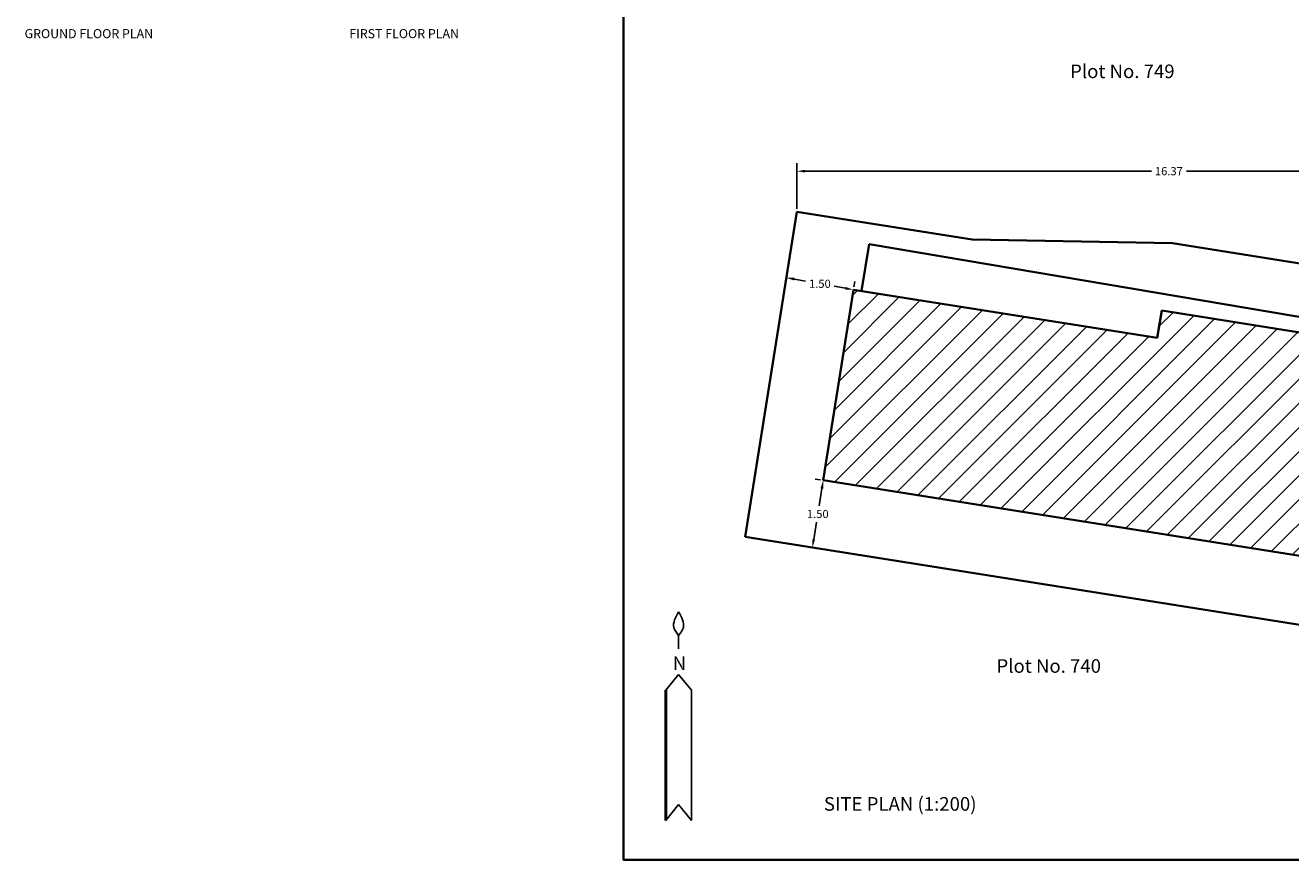
# Model space of a CAD drawing. Units: metres. Extents: x 8.1 to 56.2, y -9.3 to 36.3.
# Tile 1 of 6: x 9.4 to 37.2, y -9.3 to 9.1. Entities that reach past the tile are written whole.
import ezdxf

# ---------------------------------------------------------------- set-up
doc = ezdxf.new("R2010")
doc.units = ezdxf.units.M
doc.header["$LTSCALE"] = 0.01
doc.header["$MEASUREMENT"] = 0
for name, color, linetype, lineweight in [('A-ANNO-DIMS', 2, 'Continuous', 18), ('A-ANNO-SYMB', 1, 'Continuous', 25), ('A-ANNO-TEXT', 7, 'Continuous', 18), ('A-ANNO-TTLB', 7, 'Continuous', 35), ('A-AREA-PATT', 1, 'Continuous', 13), ('A-WALL', 7, 'Continuous', 50), ('C-BLDG', 1, 'Continuous', 35), ('C-PROP', 5, 'Continuous', 35)]:
    doc.layers.add(name, color=color, linetype=linetype, lineweight=lineweight)
doc.styles.get("Standard").update_dxf_attribs({"font": 'arial.ttf'})
doc.dimstyles.get("Standard").update_dxf_attribs({"dimtxt": 0.18, "dimasz": 0.18, "dimexe": 0.18, "dimexo": 0.0625, "dimgap": 0.09, "dimtad": 0, "dimtih": 1, "dimtoh": 1, "dimzin": 0, "dimdsep": 46, "dimtxsty": 'Standard', "dimcen": 0.09, "dimadec": 0, "dimazin": 0, "dimtfac": 1, "dimtofl": 0, "dimtmove": 0, "dimatfit": 3, "dimfxl": 1, "dimtolj": 1, "dimtzin": 0, "dimarcsym": 0})

# ---------------------------------------------------------------- blocks, each defined once
blk = doc.blocks.new('*D11')
at = {"layer": 'A-ANNO-DIMS', "color": 0, "lineweight": -2, "transparency": 16777216}
for p, q in [((26.382, 5.014), (26.382, 6.024)), ((42.755, 3.933), (42.755, 6.024)), ((26.562, 5.844), (34.183, 5.844)), ((42.575, 5.844), (34.954, 5.844))]:
    blk.add_line(p, q, dxfattribs=at)
at = {"layer": 'A-ANNO-DIMS', "color": 0, "transparency": 16777216}
for points in [[(26.562, 5.874), (26.562, 5.814), (26.382, 5.844)], [(42.575, 5.874), (42.575, 5.814), (42.755, 5.844)]]:
    blk.add_solid(points, dxfattribs=at)
at = {"layer": 'Defpoints', "color": 0, "transparency": 16777216}
for p in [(42.755, 5.844), (26.382, 4.951), (42.755, 3.87)]:
    blk.add_point(p, dxfattribs=at)
at = {"layer": 'A-ANNO-DIMS', "color": 0, "transparency": 16777216, "insert": (34.568, 5.844), "char_height": 0.18, "attachment_point": 5}
blk.add_mtext('\\A1;16.37', dxfattribs=at)
blk = doc.blocks.new('*D13')
at = {"layer": 'A-ANNO-DIMS', "color": 0, "lineweight": -2, "transparency": 16777216}
for p, q in [((26.9, -0.953), (26.784, -0.935)), ((26.933, -1.141), (26.873, -1.522)), ((26.755, -2.267), (26.815, -1.886)), ((26.665, -2.435), (26.549, -2.416))]:
    blk.add_line(p, q, dxfattribs=at)
at = {"layer": 'A-ANNO-DIMS', "color": 0, "transparency": 16777216}
for points in [[(26.904, -1.136), (26.963, -1.145), (26.962, -0.963)], [(26.725, -2.262), (26.784, -2.271), (26.726, -2.444)]]:
    blk.add_solid(points, dxfattribs=at)
at = {"layer": 'Defpoints', "color": 0, "transparency": 16777216}
for p in [(26.962, -0.963), (26.726, -2.444), (26.726, -2.444)]:
    blk.add_point(p, dxfattribs=at)
at = {"layer": 'A-ANNO-DIMS', "color": 0, "transparency": 16777216, "insert": (26.844, -1.704), "char_height": 0.18, "attachment_point": 5}
blk.add_mtext('\\A1;1.50', dxfattribs=at)
blk = doc.blocks.new('*D14')
at = {"layer": 'A-ANNO-DIMS', "color": 0, "lineweight": -2, "transparency": 16777216}
for p, q in [((26.162, 3.559), (26.183, 3.675)), ((26.328, 3.466), (26.575, 3.422)), ((27.639, 3.296), (27.66, 3.412)), ((27.451, 3.266), (27.205, 3.31))]:
    blk.add_line(p, q, dxfattribs=at)
at = {"layer": 'A-ANNO-DIMS', "color": 0, "transparency": 16777216}
for points in [[(26.334, 3.496), (26.323, 3.437), (26.151, 3.498)], [(27.456, 3.296), (27.446, 3.237), (27.628, 3.234)]]:
    blk.add_solid(points, dxfattribs=at)
at = {"layer": 'Defpoints', "color": 0, "transparency": 16777216}
for p in [(26.151, 3.498), (27.628, 3.234), (27.628, 3.234)]:
    blk.add_point(p, dxfattribs=at)
at = {"layer": 'A-ANNO-DIMS', "color": 0, "transparency": 16777216, "insert": (26.89, 3.366), "char_height": 0.18, "attachment_point": 5}
blk.add_mtext('\\A1;1.50', dxfattribs=at)

msp = doc.modelspace()

# ---------------------------------------------------------------- hatches: boundary and pattern name
at = {"layer": 'A-AREA-PATT', "transparency": 33554574}
h = msp.add_hatch(dxfattribs=at)
h.set_pattern_fill('ANSI31', color=256, scale=3)
h.set_pattern_definition([(45, (-0.34318, 4.324), (-0.265165, 0.265165), [])])
h.paths.add_polyline_path([(39.287, -2.92), (40.049, 1.88), (34.41, 2.775), (34.314, 2.173), (27.628, 3.234), (26.962, -0.963)])

# ---------------------------------------------------------------- linework, layer by layer
at = {"layer": 'A-ANNO-SYMB'}
for p, q in [((23.781, -4.67), (23.781, -4.378)), ((23.497, -5.586), (23.781, -5.237)), ((23.781, -5.237), (24.065, -5.586)), ((24.065, -5.586), (24.065, -8.452)), ((23.497, -8.452), (23.781, -8.102)), ((23.781, -8.102), (24.065, -8.452))]:
    msp.add_line(p, q, dxfattribs=at)
for points in [[(23.781, -4.378), (23.736, -4.322), (23.612, -4.164), (23.715, -3.977), (23.781, -3.857)], [(23.781, -4.378), (23.826, -4.322), (23.95, -4.164), (23.847, -3.977), (23.781, -3.857)]]:
    msp.add_open_spline(points, degree=3, knots=[0, 0, 0, 0, 0.202652, 0.5657122, 0.5657122, 0.5657122, 0.5657122], dxfattribs=at)
at = {"layer": 'A-ANNO-TTLB'}
msp.add_lwpolyline([(22.566, 9.894), (52.195, 9.894), (52.195, -9.317), (22.566, -9.317)], close=True, dxfattribs=at)
at = {"layer": 'A-WALL'}
msp.add_line((23.497, -8.452), (23.497, -5.586), dxfattribs=at)
at = {"layer": 'C-BLDG'}
for p, q in [((27.973, 4.24), (27.808, 3.206)), ((42.805, 1.724), (27.973, 4.24))]:
    msp.add_line(p, q, dxfattribs=at)
at = {"layer": 'C-PROP'}
for p, q in [((26.382, 4.951), (25.245, -2.209)), ((26.382, 4.951), (30.242, 4.338)), ((34.645, 4.257), (30.242, 4.338)), ((34.645, 4.257), (42.776, 2.966)), ((27.628, 3.234), (26.962, -0.963)), ((27.628, 3.234), (34.314, 2.173)), ((34.314, 2.173), (34.41, 2.775)), ((34.314, 2.173), (34.41, 2.775)), ((34.41, 2.775), (42.812, 1.441)), ((26.962, -0.963), (42.927, -3.498)), ((25.245, -2.209), (42.963, -5.023))]:
    msp.add_line(p, q, dxfattribs=at)

# ---------------------------------------------------------------- texts
at = {"layer": 'A-ANNO-SYMB', "insert": (23.306, -4.841), "char_height": 0.3, "attachment_point": 1}
msp.add_mtext_dynamic_manual_height_columns('\\pxqc;N', width=0.98793, gutter_width=1, heights=[0], dxfattribs=at)
at = {"layer": 'A-ANNO-TEXT', "attachment_point": 1}
for s, insert, char_height in [('\\pxqc;GROUND FLOOR PLAN', (8.776, 8.973), 0.2), ('\\pxqc;FIRST FLOOR PLAN', (15.714, 8.973), 0.2), ('\\pxqc;Plot No. 749', (31.517, 8.193), 0.3), ('\\pxqc;Plot No. 740', (29.897, -4.901), 0.3), ('\\pxqc;SITE PLAN (1:200)', (26.629, -7.938), 0.3)]:
    msp.add_mtext_dynamic_manual_height_columns(s, width=4.05553, gutter_width=1, heights=[0], dxfattribs=dict(at, insert=insert, char_height=char_height))

# ---------------------------------------------------------------- dimensions: what is measured, and where the dimension line sits
at = {"layer": 'A-ANNO-DIMS'}
dim = msp.add_linear_dim(base=(42.755, 5.844), p1=(26.382, 4.951), p2=(42.755, 3.87), dimstyle='Standard', override={"dimclrd": 0, "dimclre": 0, "dimclrt": 0}, dxfattribs=at)
dim.commit()
dim.dimension.update_dxf_attribs({"geometry": '*D11', "text_midpoint": (34.568, 5.844)})
for p1, p2, picture, middle in [((26.151, 3.498), (27.628, 3.234), '*D14', (26.89, 3.366)), ((26.962, -0.963), (26.726, -2.444), '*D13', (26.844, -1.704))]:
    dim = msp.add_aligned_dim(p1=p1, p2=p2, distance=0, dimstyle='Standard', override={"dimclrd": 0, "dimclre": 0, "dimclrt": 0}, dxfattribs=at)
    dim.commit()
    dim.dimension.update_dxf_attribs({"geometry": picture, "text_midpoint": middle})

doc.saveas('drawing.dxf')
